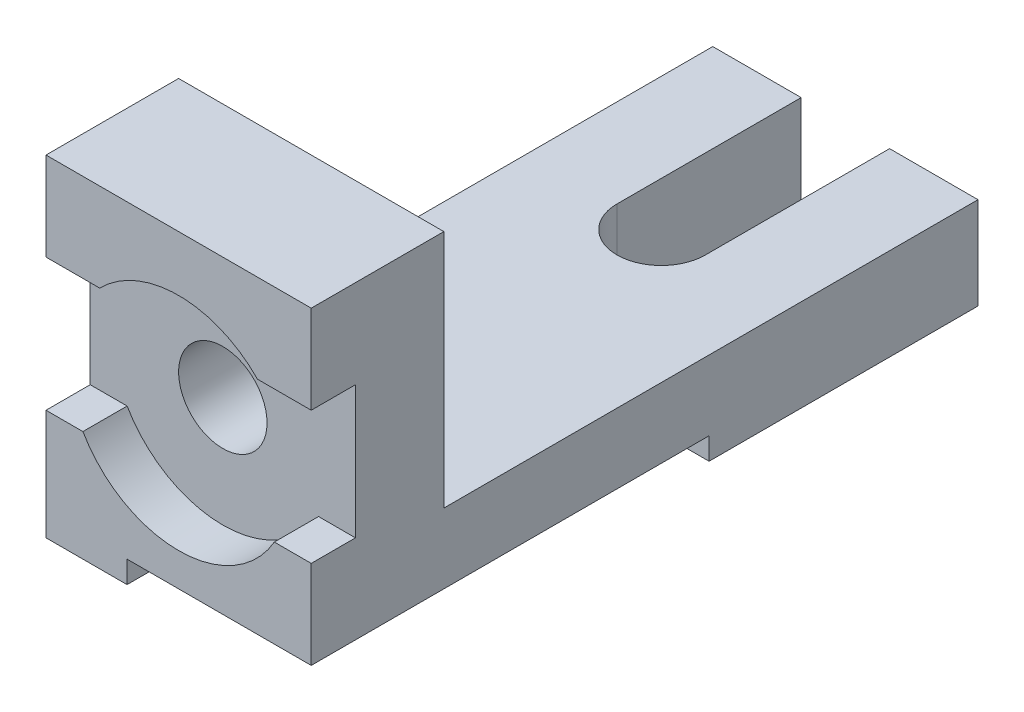
ISO-10303-21;
HEADER;
FILE_DESCRIPTION(('STEP AP214'),'2;1');
FILE_NAME('part.step','',(''),(''),'','','');
FILE_SCHEMA(('AUTOMOTIVE_DESIGN { 1 0 10303 214 1 1 1 1 }'));
ENDSEC;
DATA;
#1=APPLICATION_CONTEXT('core data for automotive mechanical design processes');
#2=APPLICATION_PROTOCOL_DEFINITION('international standard','automotive_design',2000,#1);
#3=PRODUCT_CONTEXT('',#1,'mechanical');
#4=PRODUCT('Part','Part','',(#3));
#5=PRODUCT_RELATED_PRODUCT_CATEGORY('part','',(#4));
#6=PRODUCT_DEFINITION_FORMATION('','',#4);
#7=PRODUCT_DEFINITION_CONTEXT('part definition',#1,'design');
#8=PRODUCT_DEFINITION('design','',#6,#7);
#9=PRODUCT_DEFINITION_SHAPE('','',#8);
#10=(LENGTH_UNIT() NAMED_UNIT(*) SI_UNIT(.MILLI.,.METRE.));
#11=(NAMED_UNIT(*) PLANE_ANGLE_UNIT() SI_UNIT($,.RADIAN.));
#12=(NAMED_UNIT(*) SI_UNIT($,.STERADIAN.) SOLID_ANGLE_UNIT());
#13=UNCERTAINTY_MEASURE_WITH_UNIT(LENGTH_MEASURE(1.E-05),#10,'distance_accuracy_value','');
#14=(GEOMETRIC_REPRESENTATION_CONTEXT(3) GLOBAL_UNCERTAINTY_ASSIGNED_CONTEXT((#13)) GLOBAL_UNIT_ASSIGNED_CONTEXT((#10,
#11,#12)) REPRESENTATION_CONTEXT('',''));
#15=CARTESIAN_POINT('',(0.,0.,0.));
#16=DIRECTION('',(0.,0.,1.));
#17=DIRECTION('',(1.,0.,0.));
#18=AXIS2_PLACEMENT_3D('',#15,#16,#17);
#19=CARTESIAN_POINT('',(0.,0.,-163.));
#20=DIRECTION('',(0.,0.,-1.));
#21=DIRECTION('',(-1.,0.,0.));
#22=AXIS2_PLACEMENT_3D('',#19,#20,#21);
#23=PLANE('',#22);
#24=DIRECTION('',(0.,1.,0.));
#25=VECTOR('',#24,1.);
#26=CARTESIAN_POINT('',(48.,0.,-163.));
#27=LINE('',#26,#25);
#28=CARTESIAN_POINT('',(48.,0.,-163.));
#29=VERTEX_POINT('',#28);
#30=CARTESIAN_POINT('',(48.,25.,-163.));
#31=VERTEX_POINT('',#30);
#32=EDGE_CURVE('E360',#29,#31,#27,.T.);
#33=ORIENTED_EDGE('',*,*,#32,.T.);
#34=DIRECTION('',(1.,0.,0.));
#35=VECTOR('',#34,1.);
#36=CARTESIAN_POINT('',(0.,25.,-163.));
#37=LINE('',#36,#35);
#38=CARTESIAN_POINT('',(72.,25.,-163.));
#39=VERTEX_POINT('',#38);
#40=EDGE_CURVE('E219',#31,#39,#37,.T.);
#41=ORIENTED_EDGE('',*,*,#40,.T.);
#42=DIRECTION('',(0.,1.,0.));
#43=VECTOR('',#42,1.);
#44=CARTESIAN_POINT('',(72.,0.,-163.));
#45=LINE('',#44,#43);
#46=CARTESIAN_POINT('',(72.,0.,-163.));
#47=VERTEX_POINT('',#46);
#48=EDGE_CURVE('E365',#47,#39,#45,.T.);
#49=ORIENTED_EDGE('',*,*,#48,.F.);
#50=DIRECTION('',(1.,0.,0.));
#51=VECTOR('',#50,1.);
#52=CARTESIAN_POINT('',(0.,0.,-163.));
#53=LINE('',#52,#51);
#54=EDGE_CURVE('E216',#29,#47,#53,.T.);
#55=ORIENTED_EDGE('',*,*,#54,.F.);
#56=EDGE_LOOP('',(#33,#41,#49,#55));
#57=FACE_BOUND('',#56,.T.);
#58=ADVANCED_FACE('F39',(#57),#23,.T.);
#59=CARTESIAN_POINT('',(0.,0.,-18.));
#60=DIRECTION('',(0.,0.,-1.));
#61=DIRECTION('',(-1.,0.,0.));
#62=AXIS2_PLACEMENT_3D('',#59,#60,#61);
#63=PLANE('',#62);
#64=DIRECTION('',(0.,-1.,0.));
#65=VECTOR('',#64,1.);
#66=CARTESIAN_POINT('',(0.,0.,-18.));
#67=LINE('',#66,#65);
#68=CARTESIAN_POINT('',(0.,6.,-18.));
#69=VERTEX_POINT('',#68);
#70=CARTESIAN_POINT('',(0.,0.,-18.));
#71=VERTEX_POINT('',#70);
#72=EDGE_CURVE('E305',#69,#71,#67,.T.);
#73=ORIENTED_EDGE('',*,*,#72,.F.);
#74=DIRECTION('',(1.,0.,0.));
#75=VECTOR('',#74,1.);
#76=CARTESIAN_POINT('',(0.,6.,-18.));
#77=LINE('',#76,#75);
#78=CARTESIAN_POINT('',(22.,6.,-18.));
#79=VERTEX_POINT('',#78);
#80=EDGE_CURVE('E230',#69,#79,#77,.T.);
#81=ORIENTED_EDGE('',*,*,#80,.T.);
#82=DIRECTION('',(0.,-1.,0.));
#83=VECTOR('',#82,1.);
#84=CARTESIAN_POINT('',(22.,0.,-18.));
#85=LINE('',#84,#83);
#86=CARTESIAN_POINT('',(22.,0.,-18.));
#87=VERTEX_POINT('',#86);
#88=EDGE_CURVE('E231',#79,#87,#85,.T.);
#89=ORIENTED_EDGE('',*,*,#88,.T.);
#90=DIRECTION('',(1.,0.,0.));
#91=VECTOR('',#90,1.);
#92=CARTESIAN_POINT('',(0.,0.,-18.));
#93=LINE('',#92,#91);
#94=EDGE_CURVE('E324',#71,#87,#93,.T.);
#95=ORIENTED_EDGE('',*,*,#94,.F.);
#96=EDGE_LOOP('',(#73,#81,#89,#95));
#97=FACE_BOUND('',#96,.T.);
#98=ADVANCED_FACE('F433',(#97),#63,.T.);
#99=CARTESIAN_POINT('',(0.,0.,18.));
#100=DIRECTION('',(0.,0.,-1.));
#101=DIRECTION('',(-1.,0.,0.));
#102=AXIS2_PLACEMENT_3D('',#99,#100,#101);
#103=PLANE('',#102);
#104=DIRECTION('',(0.,-1.,0.));
#105=VECTOR('',#104,1.);
#106=CARTESIAN_POINT('',(0.,0.,18.));
#107=LINE('',#106,#105);
#108=CARTESIAN_POINT('',(0.,90.,18.));
#109=VERTEX_POINT('',#108);
#110=CARTESIAN_POINT('',(0.,66.,18.));
#111=VERTEX_POINT('',#110);
#112=EDGE_CURVE('E310',#109,#111,#107,.T.);
#113=ORIENTED_EDGE('',*,*,#112,.T.);
#114=DIRECTION('',(1.,0.,0.));
#115=VECTOR('',#114,1.);
#116=CARTESIAN_POINT('',(0.,66.,18.));
#117=LINE('',#116,#115);
#118=CARTESIAN_POINT('',(14.5757147143714,66.,18.));
#119=VERTEX_POINT('',#118);
#120=EDGE_CURVE('E271',#111,#119,#117,.T.);
#121=ORIENTED_EDGE('',*,*,#120,.T.);
#122=CARTESIAN_POINT('',(36.,45.,18.));
#123=DIRECTION('',(0.,0.,1.));
#124=DIRECTION('',(1.,0.,0.));
#125=AXIS2_PLACEMENT_3D('',#122,#123,#124);
#126=CIRCLE('',#125,30.);
#127=CARTESIAN_POINT('',(57.4242852856286,66.,18.));
#128=VERTEX_POINT('',#127);
#129=EDGE_CURVE('E302',#128,#119,#126,.T.);
#130=ORIENTED_EDGE('',*,*,#129,.F.);
#131=CARTESIAN_POINT('',(72.,66.,18.));
#132=VERTEX_POINT('',#131);
#133=EDGE_CURVE('E280',#128,#132,#117,.T.);
#134=ORIENTED_EDGE('',*,*,#133,.T.);
#135=DIRECTION('',(0.,1.,0.));
#136=VECTOR('',#135,1.);
#137=CARTESIAN_POINT('',(72.,0.,18.));
#138=LINE('',#137,#136);
#139=CARTESIAN_POINT('',(72.,90.,18.));
#140=VERTEX_POINT('',#139);
#141=EDGE_CURVE('E313',#132,#140,#138,.T.);
#142=ORIENTED_EDGE('',*,*,#141,.T.);
#143=DIRECTION('',(-1.,0.,0.));
#144=VECTOR('',#143,1.);
#145=CARTESIAN_POINT('',(0.,90.,18.));
#146=LINE('',#145,#144);
#147=EDGE_CURVE('E320',#140,#109,#146,.T.);
#148=ORIENTED_EDGE('',*,*,#147,.T.);
#149=EDGE_LOOP('',(#113,#121,#130,#134,#142,#148));
#150=FACE_BOUND('',#149,.T.);
#151=ADVANCED_FACE('F457',(#150),#103,.F.);
#152=CARTESIAN_POINT('',(36.,45.,6.));
#153=DIRECTION('',(0.,0.,1.));
#154=DIRECTION('',(1.,0.,0.));
#155=AXIS2_PLACEMENT_3D('',#152,#153,#154);
#156=CYLINDRICAL_SURFACE('',#155,30.);
#157=ORIENTED_EDGE('',*,*,#129,.T.);
#158=DIRECTION('',(0.,0.,1.));
#159=VECTOR('',#158,1.);
#160=CARTESIAN_POINT('',(14.5757147143714,66.,6.));
#161=LINE('',#160,#159);
#162=CARTESIAN_POINT('',(14.5757147143714,66.,6.));
#163=VERTEX_POINT('',#162);
#164=EDGE_CURVE('E294',#119,#163,#161,.F.);
#165=ORIENTED_EDGE('',*,*,#164,.T.);
#166=CARTESIAN_POINT('',(36.,45.,6.));
#167=DIRECTION('',(0.,0.,1.));
#168=DIRECTION('',(1.,0.,0.));
#169=AXIS2_PLACEMENT_3D('',#166,#167,#168);
#170=CIRCLE('',#169,30.);
#171=CARTESIAN_POINT('',(57.4242852856286,66.,6.));
#172=VERTEX_POINT('',#171);
#173=EDGE_CURVE('E299',#172,#163,#170,.T.);
#174=ORIENTED_EDGE('',*,*,#173,.F.);
#175=DIRECTION('',(0.,0.,1.));
#176=VECTOR('',#175,1.);
#177=CARTESIAN_POINT('',(57.4242852856286,66.,6.));
#178=LINE('',#177,#176);
#179=EDGE_CURVE('E292',#172,#128,#178,.T.);
#180=ORIENTED_EDGE('',*,*,#179,.T.);
#181=EDGE_LOOP('',(#157,#165,#174,#180));
#182=FACE_BOUND('',#181,.T.);
#183=ADVANCED_FACE('F510',(#182),#156,.F.);
#184=CARTESIAN_POINT('',(0.,0.,18.));
#185=DIRECTION('',(1.,0.,0.));
#186=DIRECTION('',(0.,0.,-1.));
#187=AXIS2_PLACEMENT_3D('',#184,#185,#186);
#188=PLANE('',#187);
#189=DIRECTION('',(0.,1.,0.));
#190=VECTOR('',#189,1.);
#191=CARTESIAN_POINT('',(0.,45.,6.));
#192=LINE('',#191,#190);
#193=CARTESIAN_POINT('',(0.,30.,5.99999999999999));
#194=VERTEX_POINT('',#193);
#195=CARTESIAN_POINT('',(0.,66.,6.));
#196=VERTEX_POINT('',#195);
#197=EDGE_CURVE('E256',#194,#196,#192,.T.);
#198=ORIENTED_EDGE('',*,*,#197,.T.);
#199=DIRECTION('',(0.,0.,1.));
#200=VECTOR('',#199,1.);
#201=CARTESIAN_POINT('',(0.,66.,18.));
#202=LINE('',#201,#200);
#203=EDGE_CURVE('E264',#196,#111,#202,.T.);
#204=ORIENTED_EDGE('',*,*,#203,.T.);
#205=ORIENTED_EDGE('',*,*,#112,.F.);
#206=DIRECTION('',(0.,0.,-1.));
#207=VECTOR('',#206,1.);
#208=CARTESIAN_POINT('',(0.,90.,18.));
#209=LINE('',#208,#207);
#210=CARTESIAN_POINT('',(0.,90.,-18.));
#211=VERTEX_POINT('',#210);
#212=EDGE_CURVE('E316',#109,#211,#209,.T.);
#213=ORIENTED_EDGE('',*,*,#212,.T.);
#214=CARTESIAN_POINT('',(0.,25.,-18.));
#215=VERTEX_POINT('',#214);
#216=EDGE_CURVE('E318',#211,#215,#67,.T.);
#217=ORIENTED_EDGE('',*,*,#216,.T.);
#218=DIRECTION('',(0.,0.,1.));
#219=VECTOR('',#218,1.);
#220=CARTESIAN_POINT('',(0.,25.,-163.));
#221=LINE('',#220,#219);
#222=CARTESIAN_POINT('',(0.,25.,-163.));
#223=VERTEX_POINT('',#222);
#224=EDGE_CURVE('E235',#223,#215,#221,.T.);
#225=ORIENTED_EDGE('',*,*,#224,.F.);
#226=DIRECTION('',(0.,1.,0.));
#227=VECTOR('',#226,1.);
#228=CARTESIAN_POINT('',(0.,0.,-163.));
#229=LINE('',#228,#227);
#230=CARTESIAN_POINT('',(0.,0.,-163.));
#231=VERTEX_POINT('',#230);
#232=EDGE_CURVE('E348',#231,#223,#229,.T.);
#233=ORIENTED_EDGE('',*,*,#232,.F.);
#234=DIRECTION('',(0.,0.,-1.));
#235=VECTOR('',#234,1.);
#236=CARTESIAN_POINT('',(0.,0.,-90.));
#237=LINE('',#236,#235);
#238=CARTESIAN_POINT('',(0.,0.,-90.));
#239=VERTEX_POINT('',#238);
#240=EDGE_CURVE('E220',#239,#231,#237,.T.);
#241=ORIENTED_EDGE('',*,*,#240,.F.);
#242=DIRECTION('',(0.,-1.,0.));
#243=VECTOR('',#242,1.);
#244=CARTESIAN_POINT('',(0.,6.,-90.));
#245=LINE('',#244,#243);
#246=CARTESIAN_POINT('',(0.,6.,-90.));
#247=VERTEX_POINT('',#246);
#248=EDGE_CURVE('E368',#247,#239,#245,.T.);
#249=ORIENTED_EDGE('',*,*,#248,.F.);
#250=DIRECTION('',(0.,0.,-1.));
#251=VECTOR('',#250,1.);
#252=CARTESIAN_POINT('',(0.,6.,-18.));
#253=LINE('',#252,#251);
#254=EDGE_CURVE('E366',#69,#247,#253,.T.);
#255=ORIENTED_EDGE('',*,*,#254,.F.);
#256=ORIENTED_EDGE('',*,*,#72,.T.);
#257=DIRECTION('',(0.,0.,-1.));
#258=VECTOR('',#257,1.);
#259=CARTESIAN_POINT('',(0.,0.,18.));
#260=LINE('',#259,#258);
#261=CARTESIAN_POINT('',(0.,0.,18.));
#262=VERTEX_POINT('',#261);
#263=EDGE_CURVE('E11',#262,#71,#260,.T.);
#264=ORIENTED_EDGE('',*,*,#263,.F.);
#265=CARTESIAN_POINT('',(0.,30.,18.));
#266=VERTEX_POINT('',#265);
#267=EDGE_CURVE('E311',#266,#262,#107,.T.);
#268=ORIENTED_EDGE('',*,*,#267,.F.);
#269=DIRECTION('',(0.,0.,-1.));
#270=VECTOR('',#269,1.);
#271=CARTESIAN_POINT('',(0.,30.,5.99999999999999));
#272=LINE('',#271,#270);
#273=EDGE_CURVE('E257',#266,#194,#272,.T.);
#274=ORIENTED_EDGE('',*,*,#273,.T.);
#275=EDGE_LOOP('',(#198,#204,#205,#213,#217,#225,#233,#241,#249,#255,#256,#264,#268,#274));
#276=FACE_BOUND('',#275,.T.);
#277=ADVANCED_FACE('F41',(#276),#188,.F.);
#278=CARTESIAN_POINT('',(0.,0.,18.));
#279=DIRECTION('',(0.,1.,0.));
#280=DIRECTION('',(0.,0.,1.));
#281=AXIS2_PLACEMENT_3D('',#278,#279,#280);
#282=PLANE('',#281);
#283=ORIENTED_EDGE('',*,*,#94,.T.);
#284=DIRECTION('',(0.,0.,1.));
#285=VECTOR('',#284,1.);
#286=CARTESIAN_POINT('',(22.,0.,-18.));
#287=LINE('',#286,#285);
#288=CARTESIAN_POINT('',(22.,0.,18.));
#289=VERTEX_POINT('',#288);
#290=EDGE_CURVE('E243',#87,#289,#287,.T.);
#291=ORIENTED_EDGE('',*,*,#290,.T.);
#292=DIRECTION('',(1.,0.,0.));
#293=VECTOR('',#292,1.);
#294=CARTESIAN_POINT('',(0.,0.,18.));
#295=LINE('',#294,#293);
#296=EDGE_CURVE('E309',#262,#289,#295,.T.);
#297=ORIENTED_EDGE('',*,*,#296,.F.);
#298=ORIENTED_EDGE('',*,*,#263,.T.);
#299=EDGE_LOOP('',(#283,#291,#297,#298));
#300=FACE_BOUND('',#299,.T.);
#301=ADVANCED_FACE('F427',(#300),#282,.F.);
#302=CARTESIAN_POINT('',(72.,0.,18.));
#303=DIRECTION('',(-1.,0.,0.));
#304=DIRECTION('',(0.,0.,1.));
#305=AXIS2_PLACEMENT_3D('',#302,#303,#304);
#306=PLANE('',#305);
#307=CARTESIAN_POINT('',(72.,6.,18.));
#308=VERTEX_POINT('',#307);
#309=CARTESIAN_POINT('',(72.,30.,18.));
#310=VERTEX_POINT('',#309);
#311=EDGE_CURVE('E314',#308,#310,#138,.T.);
#312=ORIENTED_EDGE('',*,*,#311,.F.);
#313=DIRECTION('',(0.,0.,1.));
#314=VECTOR('',#313,1.);
#315=CARTESIAN_POINT('',(72.,6.,-18.));
#316=LINE('',#315,#314);
#317=CARTESIAN_POINT('',(72.,6.,-90.));
#318=VERTEX_POINT('',#317);
#319=EDGE_CURVE('E236',#318,#308,#316,.T.);
#320=ORIENTED_EDGE('',*,*,#319,.F.);
#321=DIRECTION('',(0.,-1.,0.));
#322=VECTOR('',#321,1.);
#323=CARTESIAN_POINT('',(72.,6.,-90.));
#324=LINE('',#323,#322);
#325=CARTESIAN_POINT('',(72.,0.,-90.));
#326=VERTEX_POINT('',#325);
#327=EDGE_CURVE('E353',#318,#326,#324,.T.);
#328=ORIENTED_EDGE('',*,*,#327,.T.);
#329=DIRECTION('',(0.,0.,-1.));
#330=VECTOR('',#329,1.);
#331=CARTESIAN_POINT('',(72.,0.,-90.));
#332=LINE('',#331,#330);
#333=EDGE_CURVE('E356',#326,#47,#332,.T.);
#334=ORIENTED_EDGE('',*,*,#333,.T.);
#335=ORIENTED_EDGE('',*,*,#48,.T.);
#336=DIRECTION('',(0.,0.,1.));
#337=VECTOR('',#336,1.);
#338=CARTESIAN_POINT('',(72.,25.,-163.));
#339=LINE('',#338,#337);
#340=CARTESIAN_POINT('',(72.,25.,-18.));
#341=VERTEX_POINT('',#340);
#342=EDGE_CURVE('E362',#39,#341,#339,.T.);
#343=ORIENTED_EDGE('',*,*,#342,.T.);
#344=DIRECTION('',(0.,1.,0.));
#345=VECTOR('',#344,1.);
#346=CARTESIAN_POINT('',(72.,0.,-18.));
#347=LINE('',#346,#345);
#348=CARTESIAN_POINT('',(72.,90.,-18.));
#349=VERTEX_POINT('',#348);
#350=EDGE_CURVE('E65',#341,#349,#347,.T.);
#351=ORIENTED_EDGE('',*,*,#350,.T.);
#352=DIRECTION('',(0.,0.,-1.));
#353=VECTOR('',#352,1.);
#354=CARTESIAN_POINT('',(72.,90.,18.));
#355=LINE('',#354,#353);
#356=EDGE_CURVE('E50',#140,#349,#355,.T.);
#357=ORIENTED_EDGE('',*,*,#356,.F.);
#358=ORIENTED_EDGE('',*,*,#141,.F.);
#359=DIRECTION('',(0.,0.,1.));
#360=VECTOR('',#359,1.);
#361=CARTESIAN_POINT('',(72.,66.,18.));
#362=LINE('',#361,#360);
#363=CARTESIAN_POINT('',(72.,66.,6.));
#364=VERTEX_POINT('',#363);
#365=EDGE_CURVE('E258',#364,#132,#362,.T.);
#366=ORIENTED_EDGE('',*,*,#365,.F.);
#367=DIRECTION('',(0.,1.,0.));
#368=VECTOR('',#367,1.);
#369=CARTESIAN_POINT('',(72.,66.,6.));
#370=LINE('',#369,#368);
#371=CARTESIAN_POINT('',(72.,30.,5.99999999999999));
#372=VERTEX_POINT('',#371);
#373=EDGE_CURVE('E266',#372,#364,#370,.T.);
#374=ORIENTED_EDGE('',*,*,#373,.F.);
#375=DIRECTION('',(0.,0.,-1.));
#376=VECTOR('',#375,1.);
#377=CARTESIAN_POINT('',(72.,30.,5.99999999999999));
#378=LINE('',#377,#376);
#379=EDGE_CURVE('E254',#310,#372,#378,.T.);
#380=ORIENTED_EDGE('',*,*,#379,.F.);
#381=EDGE_LOOP('',(#312,#320,#328,#334,#335,#343,#351,#357,#358,#366,#374,#380));
#382=FACE_BOUND('',#381,.T.);
#383=ADVANCED_FACE('F397',(#382),#306,.F.);
#384=CARTESIAN_POINT('',(0.,90.,18.));
#385=DIRECTION('',(0.,-1.,0.));
#386=DIRECTION('',(0.,0.,-1.));
#387=AXIS2_PLACEMENT_3D('',#384,#385,#386);
#388=PLANE('',#387);
#389=DIRECTION('',(-1.,0.,0.));
#390=VECTOR('',#389,1.);
#391=CARTESIAN_POINT('',(0.,90.,-18.));
#392=LINE('',#391,#390);
#393=EDGE_CURVE('E330',#349,#211,#392,.T.);
#394=ORIENTED_EDGE('',*,*,#393,.T.);
#395=ORIENTED_EDGE('',*,*,#212,.F.);
#396=ORIENTED_EDGE('',*,*,#147,.F.);
#397=ORIENTED_EDGE('',*,*,#356,.T.);
#398=EDGE_LOOP('',(#394,#395,#396,#397));
#399=FACE_BOUND('',#398,.T.);
#400=ADVANCED_FACE('F331',(#399),#388,.F.);
#401=ORIENTED_EDGE('',*,*,#296,.T.);
#402=DIRECTION('',(0.,-1.,0.));
#403=VECTOR('',#402,1.);
#404=CARTESIAN_POINT('',(22.,0.,18.));
#405=LINE('',#404,#403);
#406=CARTESIAN_POINT('',(22.,6.,18.));
#407=VERTEX_POINT('',#406);
#408=EDGE_CURVE('E240',#407,#289,#405,.T.);
#409=ORIENTED_EDGE('',*,*,#408,.F.);
#410=DIRECTION('',(-1.,0.,0.));
#411=VECTOR('',#410,1.);
#412=CARTESIAN_POINT('',(22.,6.,18.));
#413=LINE('',#412,#411);
#414=EDGE_CURVE('E238',#308,#407,#413,.T.);
#415=ORIENTED_EDGE('',*,*,#414,.F.);
#416=ORIENTED_EDGE('',*,*,#311,.T.);
#417=DIRECTION('',(1.,0.,0.));
#418=VECTOR('',#417,1.);
#419=CARTESIAN_POINT('',(0.,30.,18.));
#420=LINE('',#419,#418);
#421=CARTESIAN_POINT('',(61.9807621135332,30.,18.));
#422=VERTEX_POINT('',#421);
#423=EDGE_CURVE('E267',#422,#310,#420,.T.);
#424=ORIENTED_EDGE('',*,*,#423,.F.);
#425=CARTESIAN_POINT('',(10.0192378864668,30.,18.));
#426=VERTEX_POINT('',#425);
#427=EDGE_CURVE('E296',#426,#422,#126,.T.);
#428=ORIENTED_EDGE('',*,*,#427,.F.);
#429=EDGE_CURVE('E283',#266,#426,#420,.T.);
#430=ORIENTED_EDGE('',*,*,#429,.F.);
#431=ORIENTED_EDGE('',*,*,#267,.T.);
#432=EDGE_LOOP('',(#401,#409,#415,#416,#424,#428,#430,#431));
#433=FACE_BOUND('',#432,.T.);
#434=ADVANCED_FACE('F403',(#433),#103,.F.);
#435=DIRECTION('',(1.,0.,0.));
#436=VECTOR('',#435,1.);
#437=CARTESIAN_POINT('',(0.,25.,-18.));
#438=LINE('',#437,#436);
#439=EDGE_CURVE('E241',#215,#341,#438,.T.);
#440=ORIENTED_EDGE('',*,*,#439,.F.);
#441=ORIENTED_EDGE('',*,*,#216,.F.);
#442=ORIENTED_EDGE('',*,*,#393,.F.);
#443=ORIENTED_EDGE('',*,*,#350,.F.);
#444=EDGE_LOOP('',(#440,#441,#442,#443));
#445=FACE_BOUND('',#444,.T.);
#446=CARTESIAN_POINT('',(36.,45.,-18.));
#447=DIRECTION('',(0.,0.,1.));
#448=DIRECTION('',(1.,0.,0.));
#449=AXIS2_PLACEMENT_3D('',#446,#447,#448);
#450=CIRCLE('',#449,12.);
#451=CARTESIAN_POINT('',(48.,45.,-18.));
#452=VERTEX_POINT('',#451);
#453=EDGE_CURVE('E249',#452,#452,#450,.T.);
#454=ORIENTED_EDGE('',*,*,#453,.T.);
#455=EDGE_LOOP('',(#454));
#456=FACE_BOUND('',#455,.T.);
#457=ADVANCED_FACE('F339',(#445,#456),#63,.T.);
#458=ORIENTED_EDGE('',*,*,#427,.T.);
#459=DIRECTION('',(0.,0.,1.));
#460=VECTOR('',#459,1.);
#461=CARTESIAN_POINT('',(61.9807621135332,30.,6.));
#462=LINE('',#461,#460);
#463=CARTESIAN_POINT('',(61.9807621135332,30.,6.));
#464=VERTEX_POINT('',#463);
#465=EDGE_CURVE('E286',#422,#464,#462,.F.);
#466=ORIENTED_EDGE('',*,*,#465,.T.);
#467=CARTESIAN_POINT('',(10.0192378864668,30.,5.99999999999999));
#468=VERTEX_POINT('',#467);
#469=EDGE_CURVE('E303',#468,#464,#170,.T.);
#470=ORIENTED_EDGE('',*,*,#469,.F.);
#471=DIRECTION('',(0.,0.,1.));
#472=VECTOR('',#471,1.);
#473=CARTESIAN_POINT('',(10.0192378864668,30.,6.));
#474=LINE('',#473,#472);
#475=EDGE_CURVE('E277',#468,#426,#474,.T.);
#476=ORIENTED_EDGE('',*,*,#475,.T.);
#477=EDGE_LOOP('',(#458,#466,#470,#476));
#478=FACE_BOUND('',#477,.T.);
#479=ADVANCED_FACE('F420',(#478),#156,.F.);
#480=CARTESIAN_POINT('',(36.,45.,6.));
#481=DIRECTION('',(0.,0.,1.));
#482=DIRECTION('',(1.,0.,0.));
#483=AXIS2_PLACEMENT_3D('',#480,#481,#482);
#484=PLANE('',#483);
#485=CARTESIAN_POINT('',(36.,45.,6.));
#486=DIRECTION('',(0.,0.,1.));
#487=DIRECTION('',(1.,0.,0.));
#488=AXIS2_PLACEMENT_3D('',#485,#486,#487);
#489=CIRCLE('',#488,12.);
#490=CARTESIAN_POINT('',(48.,45.,6.));
#491=VERTEX_POINT('',#490);
#492=EDGE_CURVE('E246',#491,#491,#489,.T.);
#493=ORIENTED_EDGE('',*,*,#492,.F.);
#494=EDGE_LOOP('',(#493));
#495=FACE_BOUND('',#494,.T.);
#496=ORIENTED_EDGE('',*,*,#469,.T.);
#497=DIRECTION('',(1.,0.,0.));
#498=VECTOR('',#497,1.);
#499=CARTESIAN_POINT('',(0.,30.,5.99999999999999));
#500=LINE('',#499,#498);
#501=EDGE_CURVE('E281',#464,#372,#500,.T.);
#502=ORIENTED_EDGE('',*,*,#501,.T.);
#503=ORIENTED_EDGE('',*,*,#373,.T.);
#504=DIRECTION('',(1.,0.,0.));
#505=VECTOR('',#504,1.);
#506=CARTESIAN_POINT('',(0.,66.,6.));
#507=LINE('',#506,#505);
#508=EDGE_CURVE('E278',#172,#364,#507,.T.);
#509=ORIENTED_EDGE('',*,*,#508,.F.);
#510=ORIENTED_EDGE('',*,*,#173,.T.);
#511=EDGE_CURVE('E279',#196,#163,#507,.T.);
#512=ORIENTED_EDGE('',*,*,#511,.F.);
#513=ORIENTED_EDGE('',*,*,#197,.F.);
#514=EDGE_CURVE('E282',#194,#468,#500,.T.);
#515=ORIENTED_EDGE('',*,*,#514,.T.);
#516=EDGE_LOOP('',(#496,#502,#503,#509,#510,#512,#513,#515));
#517=FACE_BOUND('',#516,.T.);
#518=ADVANCED_FACE('F425',(#495,#517),#484,.T.);
#519=CARTESIAN_POINT('',(0.,30.,5.99999999999999));
#520=DIRECTION('',(0.,-1.,0.));
#521=DIRECTION('',(0.,0.,-1.));
#522=AXIS2_PLACEMENT_3D('',#519,#520,#521);
#523=PLANE('',#522);
#524=ORIENTED_EDGE('',*,*,#514,.F.);
#525=ORIENTED_EDGE('',*,*,#273,.F.);
#526=ORIENTED_EDGE('',*,*,#429,.T.);
#527=ORIENTED_EDGE('',*,*,#475,.F.);
#528=EDGE_LOOP('',(#524,#525,#526,#527));
#529=FACE_BOUND('',#528,.T.);
#530=ADVANCED_FACE('F423',(#529),#523,.F.);
#531=CARTESIAN_POINT('',(0.,66.,18.));
#532=DIRECTION('',(0.,1.,0.));
#533=DIRECTION('',(0.,0.,1.));
#534=AXIS2_PLACEMENT_3D('',#531,#532,#533);
#535=PLANE('',#534);
#536=ORIENTED_EDGE('',*,*,#120,.F.);
#537=ORIENTED_EDGE('',*,*,#203,.F.);
#538=ORIENTED_EDGE('',*,*,#511,.T.);
#539=ORIENTED_EDGE('',*,*,#164,.F.);
#540=EDGE_LOOP('',(#536,#537,#538,#539));
#541=FACE_BOUND('',#540,.T.);
#542=ADVANCED_FACE('F577',(#541),#535,.F.);
#543=ORIENTED_EDGE('',*,*,#508,.T.);
#544=ORIENTED_EDGE('',*,*,#365,.T.);
#545=ORIENTED_EDGE('',*,*,#133,.F.);
#546=ORIENTED_EDGE('',*,*,#179,.F.);
#547=EDGE_LOOP('',(#543,#544,#545,#546));
#548=FACE_BOUND('',#547,.T.);
#549=ADVANCED_FACE('F568',(#548),#535,.F.);
#550=ORIENTED_EDGE('',*,*,#423,.T.);
#551=ORIENTED_EDGE('',*,*,#379,.T.);
#552=ORIENTED_EDGE('',*,*,#501,.F.);
#553=ORIENTED_EDGE('',*,*,#465,.F.);
#554=EDGE_LOOP('',(#550,#551,#552,#553));
#555=FACE_BOUND('',#554,.T.);
#556=ADVANCED_FACE('F415',(#555),#523,.F.);
#557=CARTESIAN_POINT('',(36.,45.,-18.));
#558=DIRECTION('',(0.,0.,1.));
#559=DIRECTION('',(1.,0.,0.));
#560=AXIS2_PLACEMENT_3D('',#557,#558,#559);
#561=CYLINDRICAL_SURFACE('',#560,12.);
#562=ORIENTED_EDGE('',*,*,#453,.F.);
#563=EDGE_LOOP('',(#562));
#564=FACE_BOUND('',#563,.T.);
#565=ORIENTED_EDGE('',*,*,#492,.T.);
#566=EDGE_LOOP('',(#565));
#567=FACE_BOUND('',#566,.T.);
#568=ADVANCED_FACE('F438',(#564,#567),#561,.F.);
#569=CARTESIAN_POINT('',(22.,0.,-18.));
#570=DIRECTION('',(-1.,0.,0.));
#571=DIRECTION('',(0.,0.,1.));
#572=AXIS2_PLACEMENT_3D('',#569,#570,#571);
#573=PLANE('',#572);
#574=ORIENTED_EDGE('',*,*,#408,.T.);
#575=ORIENTED_EDGE('',*,*,#290,.F.);
#576=ORIENTED_EDGE('',*,*,#88,.F.);
#577=DIRECTION('',(0.,0.,1.));
#578=VECTOR('',#577,1.);
#579=CARTESIAN_POINT('',(22.,6.,-18.));
#580=LINE('',#579,#578);
#581=EDGE_CURVE('E250',#79,#407,#580,.T.);
#582=ORIENTED_EDGE('',*,*,#581,.T.);
#583=EDGE_LOOP('',(#574,#575,#576,#582));
#584=FACE_BOUND('',#583,.T.);
#585=ADVANCED_FACE('F436',(#584),#573,.F.);
#586=CARTESIAN_POINT('',(22.,6.,-18.));
#587=DIRECTION('',(0.,1.,0.));
#588=DIRECTION('',(0.,0.,1.));
#589=AXIS2_PLACEMENT_3D('',#586,#587,#588);
#590=PLANE('',#589);
#591=ORIENTED_EDGE('',*,*,#414,.T.);
#592=ORIENTED_EDGE('',*,*,#581,.F.);
#593=ORIENTED_EDGE('',*,*,#80,.F.);
#594=ORIENTED_EDGE('',*,*,#254,.T.);
#595=DIRECTION('',(1.,0.,0.));
#596=VECTOR('',#595,1.);
#597=CARTESIAN_POINT('',(0.,6.,-90.));
#598=LINE('',#597,#596);
#599=EDGE_CURVE('E228',#247,#318,#598,.T.);
#600=ORIENTED_EDGE('',*,*,#599,.T.);
#601=ORIENTED_EDGE('',*,*,#319,.T.);
#602=EDGE_LOOP('',(#591,#592,#593,#594,#600,#601));
#603=FACE_BOUND('',#602,.T.);
#604=ADVANCED_FACE('F402',(#603),#590,.F.);
#605=CARTESIAN_POINT('',(0.,25.,-163.));
#606=DIRECTION('',(0.,1.,0.));
#607=DIRECTION('',(0.,0.,1.));
#608=AXIS2_PLACEMENT_3D('',#605,#606,#607);
#609=PLANE('',#608);
#610=DIRECTION('',(0.,0.,-1.));
#611=VECTOR('',#610,1.);
#612=CARTESIAN_POINT('',(48.,25.,-163.));
#613=LINE('',#612,#611);
#614=CARTESIAN_POINT('',(48.,25.,-113.));
#615=VERTEX_POINT('',#614);
#616=EDGE_CURVE('E205',#615,#31,#613,.T.);
#617=ORIENTED_EDGE('',*,*,#616,.F.);
#618=CARTESIAN_POINT('',(36.,25.,-113.));
#619=DIRECTION('',(0.,1.,0.));
#620=DIRECTION('',(0.,0.,1.));
#621=AXIS2_PLACEMENT_3D('',#618,#619,#620);
#622=CIRCLE('',#621,12.);
#623=CARTESIAN_POINT('',(24.,25.,-113.));
#624=VERTEX_POINT('',#623);
#625=EDGE_CURVE('E385',#624,#615,#622,.T.);
#626=ORIENTED_EDGE('',*,*,#625,.F.);
#627=DIRECTION('',(0.,0.,1.));
#628=VECTOR('',#627,1.);
#629=CARTESIAN_POINT('',(24.,25.,-163.));
#630=LINE('',#629,#628);
#631=CARTESIAN_POINT('',(24.,25.,-163.));
#632=VERTEX_POINT('',#631);
#633=EDGE_CURVE('E383',#632,#624,#630,.T.);
#634=ORIENTED_EDGE('',*,*,#633,.F.);
#635=EDGE_CURVE('E208',#223,#632,#37,.T.);
#636=ORIENTED_EDGE('',*,*,#635,.F.);
#637=ORIENTED_EDGE('',*,*,#224,.T.);
#638=ORIENTED_EDGE('',*,*,#439,.T.);
#639=ORIENTED_EDGE('',*,*,#342,.F.);
#640=ORIENTED_EDGE('',*,*,#40,.F.);
#641=EDGE_LOOP('',(#617,#626,#634,#636,#637,#638,#639,#640));
#642=FACE_BOUND('',#641,.T.);
#643=ADVANCED_FACE('F350',(#642),#609,.T.);
#644=DIRECTION('',(0.,1.,0.));
#645=VECTOR('',#644,1.);
#646=CARTESIAN_POINT('',(24.,0.,-163.));
#647=LINE('',#646,#645);
#648=CARTESIAN_POINT('',(24.,0.,-163.));
#649=VERTEX_POINT('',#648);
#650=EDGE_CURVE('E200',#649,#632,#647,.T.);
#651=ORIENTED_EDGE('',*,*,#650,.F.);
#652=EDGE_CURVE('E206',#231,#649,#53,.T.);
#653=ORIENTED_EDGE('',*,*,#652,.F.);
#654=ORIENTED_EDGE('',*,*,#232,.T.);
#655=ORIENTED_EDGE('',*,*,#635,.T.);
#656=EDGE_LOOP('',(#651,#653,#654,#655));
#657=FACE_BOUND('',#656,.T.);
#658=ADVANCED_FACE('F207',(#657),#23,.T.);
#659=CARTESIAN_POINT('',(0.,0.,-90.));
#660=DIRECTION('',(0.,-1.,0.));
#661=DIRECTION('',(0.,0.,-1.));
#662=AXIS2_PLACEMENT_3D('',#659,#660,#661);
#663=PLANE('',#662);
#664=DIRECTION('',(0.,0.,-1.));
#665=VECTOR('',#664,1.);
#666=CARTESIAN_POINT('',(48.,0.,-163.));
#667=LINE('',#666,#665);
#668=CARTESIAN_POINT('',(48.,0.,-113.));
#669=VERTEX_POINT('',#668);
#670=EDGE_CURVE('E212',#669,#29,#667,.T.);
#671=ORIENTED_EDGE('',*,*,#670,.T.);
#672=ORIENTED_EDGE('',*,*,#54,.T.);
#673=ORIENTED_EDGE('',*,*,#333,.F.);
#674=DIRECTION('',(1.,0.,0.));
#675=VECTOR('',#674,1.);
#676=CARTESIAN_POINT('',(0.,0.,-90.));
#677=LINE('',#676,#675);
#678=EDGE_CURVE('E225',#239,#326,#677,.T.);
#679=ORIENTED_EDGE('',*,*,#678,.F.);
#680=ORIENTED_EDGE('',*,*,#240,.T.);
#681=ORIENTED_EDGE('',*,*,#652,.T.);
#682=DIRECTION('',(0.,0.,1.));
#683=VECTOR('',#682,1.);
#684=CARTESIAN_POINT('',(24.,0.,-163.));
#685=LINE('',#684,#683);
#686=CARTESIAN_POINT('',(24.,0.,-113.));
#687=VERTEX_POINT('',#686);
#688=EDGE_CURVE('E194',#649,#687,#685,.T.);
#689=ORIENTED_EDGE('',*,*,#688,.T.);
#690=CARTESIAN_POINT('',(36.,0.,-113.));
#691=DIRECTION('',(0.,1.,0.));
#692=DIRECTION('',(0.,0.,1.));
#693=AXIS2_PLACEMENT_3D('',#690,#691,#692);
#694=CIRCLE('',#693,12.);
#695=EDGE_CURVE('E53',#687,#669,#694,.T.);
#696=ORIENTED_EDGE('',*,*,#695,.T.);
#697=EDGE_LOOP('',(#671,#672,#673,#679,#680,#681,#689,#696));
#698=FACE_BOUND('',#697,.T.);
#699=ADVANCED_FACE('F213',(#698),#663,.T.);
#700=CARTESIAN_POINT('',(0.,6.,-90.));
#701=DIRECTION('',(0.,0.,1.));
#702=DIRECTION('',(1.,0.,0.));
#703=AXIS2_PLACEMENT_3D('',#700,#701,#702);
#704=PLANE('',#703);
#705=ORIENTED_EDGE('',*,*,#327,.F.);
#706=ORIENTED_EDGE('',*,*,#599,.F.);
#707=ORIENTED_EDGE('',*,*,#248,.T.);
#708=ORIENTED_EDGE('',*,*,#678,.T.);
#709=EDGE_LOOP('',(#705,#706,#707,#708));
#710=FACE_BOUND('',#709,.T.);
#711=ADVANCED_FACE('F398',(#710),#704,.T.);
#712=CARTESIAN_POINT('',(48.,0.,-163.));
#713=DIRECTION('',(1.,0.,0.));
#714=DIRECTION('',(0.,0.,-1.));
#715=AXIS2_PLACEMENT_3D('',#712,#713,#714);
#716=PLANE('',#715);
#717=ORIENTED_EDGE('',*,*,#616,.T.);
#718=ORIENTED_EDGE('',*,*,#32,.F.);
#719=ORIENTED_EDGE('',*,*,#670,.F.);
#720=DIRECTION('',(0.,1.,0.));
#721=VECTOR('',#720,1.);
#722=CARTESIAN_POINT('',(48.,0.,-113.));
#723=LINE('',#722,#721);
#724=EDGE_CURVE('E380',#669,#615,#723,.T.);
#725=ORIENTED_EDGE('',*,*,#724,.T.);
#726=EDGE_LOOP('',(#717,#718,#719,#725));
#727=FACE_BOUND('',#726,.T.);
#728=ADVANCED_FACE('F475',(#727),#716,.F.);
#729=CARTESIAN_POINT('',(36.,0.,-113.));
#730=DIRECTION('',(0.,1.,0.));
#731=DIRECTION('',(0.,0.,1.));
#732=AXIS2_PLACEMENT_3D('',#729,#730,#731);
#733=CYLINDRICAL_SURFACE('',#732,12.);
#734=ORIENTED_EDGE('',*,*,#625,.T.);
#735=ORIENTED_EDGE('',*,*,#724,.F.);
#736=ORIENTED_EDGE('',*,*,#695,.F.);
#737=DIRECTION('',(0.,1.,0.));
#738=VECTOR('',#737,1.);
#739=CARTESIAN_POINT('',(24.,0.,-113.));
#740=LINE('',#739,#738);
#741=EDGE_CURVE('E196',#687,#624,#740,.T.);
#742=ORIENTED_EDGE('',*,*,#741,.T.);
#743=EDGE_LOOP('',(#734,#735,#736,#742));
#744=FACE_BOUND('',#743,.T.);
#745=ADVANCED_FACE('F469',(#744),#733,.F.);
#746=CARTESIAN_POINT('',(24.,0.,-163.));
#747=DIRECTION('',(-1.,0.,0.));
#748=DIRECTION('',(0.,0.,1.));
#749=AXIS2_PLACEMENT_3D('',#746,#747,#748);
#750=PLANE('',#749);
#751=ORIENTED_EDGE('',*,*,#633,.T.);
#752=ORIENTED_EDGE('',*,*,#741,.F.);
#753=ORIENTED_EDGE('',*,*,#688,.F.);
#754=ORIENTED_EDGE('',*,*,#650,.T.);
#755=EDGE_LOOP('',(#751,#752,#753,#754));
#756=FACE_BOUND('',#755,.T.);
#757=ADVANCED_FACE('F197',(#756),#750,.F.);
#758=CLOSED_SHELL('',(#58,#98,#151,#183,#277,#301,#383,#400,#434,#457,#479,#518,#530,#542,#549,
#556,#568,#585,#604,#643,#658,#699,#711,#728,#745,#757));
#759=MANIFOLD_SOLID_BREP('B2',#758);
#760=ADVANCED_BREP_SHAPE_REPRESENTATION('',(#18,#759),#14);
#761=SHAPE_DEFINITION_REPRESENTATION(#9,#760);
ENDSEC;
END-ISO-10303-21;
